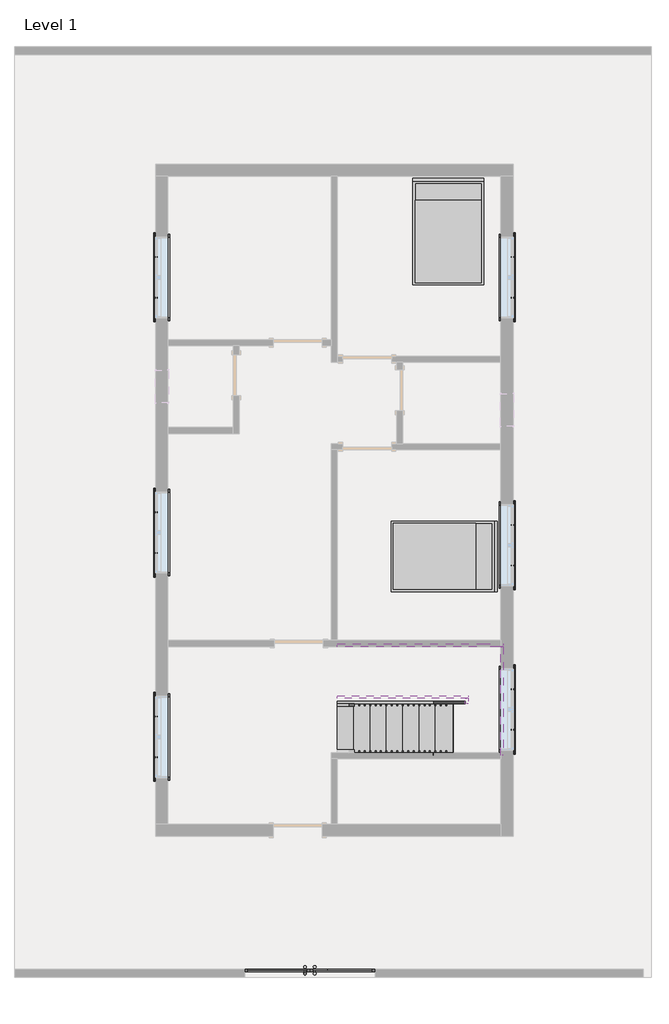
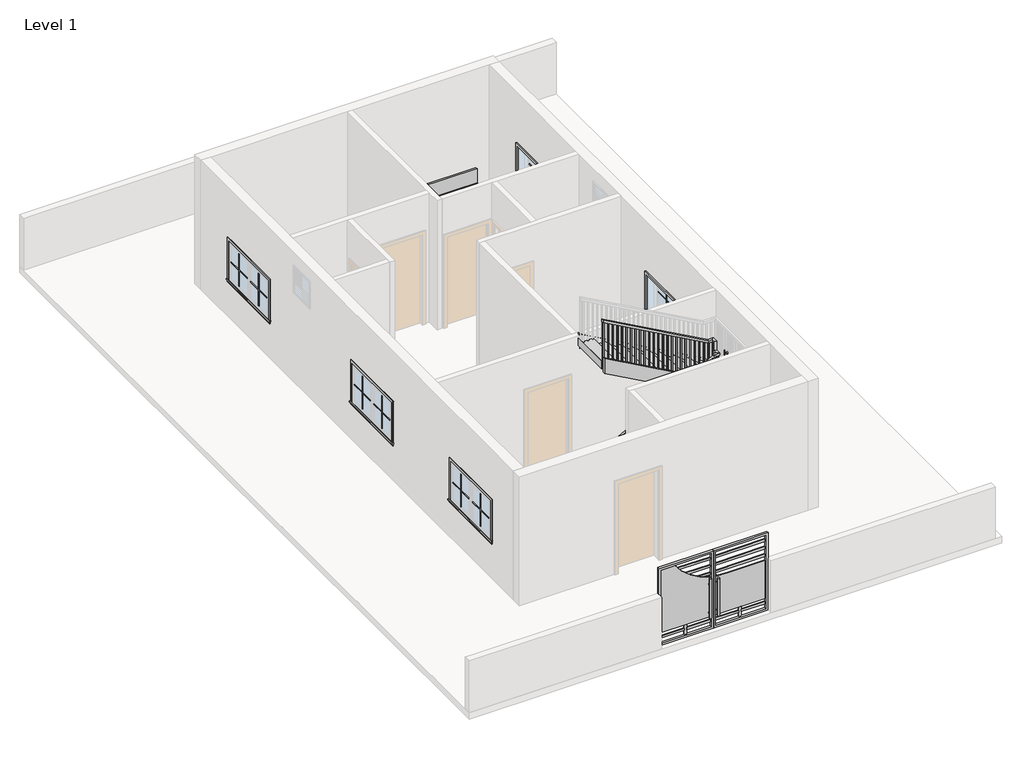
# One storey, part 3 of 3: 25 proxies, 6 members, 2 furniture elements, 1 railing, 1 stair flight.
"""IFC4 building model written with IfcOpenShell, lengths in millimetres."""

from ifc_helpers import new_model, si_unit, frame, origin, place, context, project, spatial, polyline, outline, extrude, faceted_brep, transform, mapped, element, save
from components import generic_models_113f6068, muntin_pattern_2x2_muntin_pattern_2x2_9352d081, muntin_pattern_2x2_muntin_pattern_2x2_5c2cbe28, trim_window_exterior_flat_with_sill_979bde60, trim_window_interior_flat_picture_frame_7883d11b, bed_17739_bed_17739_15c61121, stair_flight_11d7aa5f

model = new_model("IFC4")

# Units and contexts
model_context = context("Model", 3, world=origin())
ifc_project = project(units=[si_unit("LENGTHUNIT", "METRE", prefix="MILLI")], contexts=[model_context])

# Site, building, storey
site = spatial("IfcSite", under=ifc_project)
building = spatial("IfcBuilding", under=site)
storey = spatial("IfcBuildingStorey", under=building, Name="Level 1", Elevation=0.0)

# Proxies
placement = place(None, origin())
generic_models_shape = generic_models_113f6068(model_context)
element("IfcBuildingElementProxy", 1, Name="Generic Models", at=placement, inside=storey, context=model_context, shape_type="MappedRepresentation", body=[
    mapped(generic_models_shape, transform((-1712.32188, -8858.1500287, 0.0), x_axis=(1.0, 0.0, 0.0), y_axis=(0.0, 1.0, 0.0), z_axis=(0.0, 0.0, 1.0))),
])
muntin_pattern_2x2_muntin_pattern_2x2_shape = muntin_pattern_2x2_muntin_pattern_2x2_9352d081(model_context)
element("IfcBuildingElementProxy", 2, Name="Muntin Pattern_2x2 : Muntin Pattern_2x2", ObjectType="Muntin Pattern_2x2 : Muntin Pattern_2x2", at=placement, inside=storey, context=model_context, shape_type="MappedRepresentation", body=[
    mapped(muntin_pattern_2x2_muntin_pattern_2x2_shape, transform((-4579.34688, 3675.02881, 984.25), x_axis=(0.0, 1.0, 0.0), y_axis=(-1.0, 0.0, 0.0), z_axis=(0.0, 0.0, 1.0))),
])
element("IfcBuildingElementProxy", 3, Name="Muntin Pattern_2x2 : Muntin Pattern_2x2", ObjectType="Muntin Pattern_2x2 : Muntin Pattern_2x2", at=placement, inside=storey, context=model_context, shape_type="MappedRepresentation", body=[
    mapped(muntin_pattern_2x2_muntin_pattern_2x2_shape, transform((-4579.34688, -1087.47119, 984.25), x_axis=(0.0, 1.0, 0.0), y_axis=(-1.0, 0.0, 0.0), z_axis=(0.0, 0.0, 1.0))),
])
element("IfcBuildingElementProxy", 4, Name="Muntin Pattern_2x2 : Muntin Pattern_2x2", ObjectType="Muntin Pattern_2x2 : Muntin Pattern_2x2", at=placement, inside=storey, context=model_context, shape_type="MappedRepresentation", body=[
    mapped(muntin_pattern_2x2_muntin_pattern_2x2_shape, transform((-4579.34688, -4900.64619, 984.25), x_axis=(0.0, 1.0, 0.0), y_axis=(-1.0, 0.0, 0.0), z_axis=(0.0, 0.0, 1.0))),
])
element("IfcBuildingElementProxy", 5, Name="Muntin Pattern_2x2 : Muntin Pattern_2x2", ObjectType="Muntin Pattern_2x2 : Muntin Pattern_2x2", at=placement, inside=storey, context=model_context, shape_type="MappedRepresentation", body=[
    mapped(muntin_pattern_2x2_muntin_pattern_2x2_shape, transform((2069.10312, -3630.64619, 984.25), x_axis=(0.0, -1.0, 0.0), y_axis=(1.0, 0.0, 0.0), z_axis=(0.0, 0.0, 1.0))),
])
element("IfcBuildingElementProxy", 6, Name="Muntin Pattern_2x2 : Muntin Pattern_2x2", ObjectType="Muntin Pattern_2x2 : Muntin Pattern_2x2", at=placement, inside=storey, context=model_context, shape_type="MappedRepresentation", body=[
    mapped(muntin_pattern_2x2_muntin_pattern_2x2_shape, transform((2069.10312, 4433.85381, 984.25), x_axis=(0.0, -1.0, 0.0), y_axis=(1.0, 0.0, 0.0), z_axis=(0.0, 0.0, 1.0))),
])
element("IfcBuildingElementProxy", 7, Name="Muntin Pattern_2x2 : Muntin Pattern_2x2", ObjectType="Muntin Pattern_2x2 : Muntin Pattern_2x2", at=placement, inside=storey, context=model_context, shape_type="MappedRepresentation", body=[
    mapped(muntin_pattern_2x2_muntin_pattern_2x2_shape, transform((2069.10312, -563.59619, 984.25), x_axis=(0.0, -1.0, 0.0), y_axis=(1.0, 0.0, 0.0), z_axis=(0.0, 0.0, 1.0))),
])
muntin_pattern_2x2_muntin_pattern_2x2_2_shape = muntin_pattern_2x2_muntin_pattern_2x2_5c2cbe28(model_context)
element("IfcBuildingElementProxy", 8, Name="Muntin Pattern_2x2 : Muntin Pattern_2x2", ObjectType="Muntin Pattern_2x2 : Muntin Pattern_2x2", at=placement, inside=storey, context=model_context, shape_type="MappedRepresentation", body=[
    mapped(muntin_pattern_2x2_muntin_pattern_2x2_2_shape, transform((-4579.34688, 4433.85381, 984.25), x_axis=(0.0, -1.0, 0.0), y_axis=(1.0, 0.0, 0.0), z_axis=(0.0, 0.0, 1.0))),
])
element("IfcBuildingElementProxy", 9, Name="Muntin Pattern_2x2 : Muntin Pattern_2x2", ObjectType="Muntin Pattern_2x2 : Muntin Pattern_2x2", at=placement, inside=storey, context=model_context, shape_type="MappedRepresentation", body=[
    mapped(muntin_pattern_2x2_muntin_pattern_2x2_2_shape, transform((-4579.34688, -328.64619, 984.25), x_axis=(0.0, -1.0, 0.0), y_axis=(1.0, 0.0, 0.0), z_axis=(0.0, 0.0, 1.0))),
])
element("IfcBuildingElementProxy", 10, Name="Muntin Pattern_2x2 : Muntin Pattern_2x2", ObjectType="Muntin Pattern_2x2 : Muntin Pattern_2x2", at=placement, inside=storey, context=model_context, shape_type="MappedRepresentation", body=[
    mapped(muntin_pattern_2x2_muntin_pattern_2x2_2_shape, transform((-4579.34688, -4141.82119, 984.25), x_axis=(0.0, -1.0, 0.0), y_axis=(1.0, 0.0, 0.0), z_axis=(0.0, 0.0, 1.0))),
])
element("IfcBuildingElementProxy", 11, Name="Muntin Pattern_2x2 : Muntin Pattern_2x2", ObjectType="Muntin Pattern_2x2 : Muntin Pattern_2x2", at=placement, inside=storey, context=model_context, shape_type="MappedRepresentation", body=[
    mapped(muntin_pattern_2x2_muntin_pattern_2x2_2_shape, transform((2069.10312, -4389.47119, 984.25), x_axis=(0.0, 1.0, 0.0), y_axis=(-1.0, 0.0, 0.0), z_axis=(0.0, 0.0, 1.0))),
])
element("IfcBuildingElementProxy", 12, Name="Muntin Pattern_2x2 : Muntin Pattern_2x2", ObjectType="Muntin Pattern_2x2 : Muntin Pattern_2x2", at=placement, inside=storey, context=model_context, shape_type="MappedRepresentation", body=[
    mapped(muntin_pattern_2x2_muntin_pattern_2x2_2_shape, transform((2069.10312, 3675.02881, 984.25), x_axis=(0.0, 1.0, 0.0), y_axis=(-1.0, 0.0, 0.0), z_axis=(0.0, 0.0, 1.0))),
])
element("IfcBuildingElementProxy", 13, Name="Muntin Pattern_2x2 : Muntin Pattern_2x2", ObjectType="Muntin Pattern_2x2 : Muntin Pattern_2x2", at=placement, inside=storey, context=model_context, shape_type="MappedRepresentation", body=[
    mapped(muntin_pattern_2x2_muntin_pattern_2x2_2_shape, transform((2069.10312, -1322.42119, 984.25), x_axis=(0.0, 1.0, 0.0), y_axis=(-1.0, 0.0, 0.0), z_axis=(0.0, 0.0, 1.0))),
])
trim_window_exterior_flat_with_sill_shape = trim_window_exterior_flat_with_sill_979bde60(model_context)
element("IfcBuildingElementProxy", 14, Name="Trim-Window-Exterior-Flat : with Sill", ObjectType="Trim-Window-Exterior-Flat : with Sill", at=placement, inside=storey, context=model_context, shape_type="MappedRepresentation", body=[
    mapped(trim_window_exterior_flat_with_sill_shape, transform((-4588.87188, 4054.44131, 1828.8), x_axis=(0.0, -1.0, 0.0), y_axis=(0.0, 0.0, 1.0), z_axis=(-1.0, 0.0, 0.0))),
])
element("IfcBuildingElementProxy", 15, Name="Trim-Window-Exterior-Flat : with Sill", ObjectType="Trim-Window-Exterior-Flat : with Sill", at=placement, inside=storey, context=model_context, shape_type="MappedRepresentation", body=[
    mapped(trim_window_exterior_flat_with_sill_shape, transform((-4588.87188, -708.05869, 1828.8), x_axis=(0.0, -1.0, 0.0), y_axis=(0.0, 0.0, 1.0), z_axis=(-1.0, 0.0, 0.0))),
])
element("IfcBuildingElementProxy", 16, Name="Trim-Window-Exterior-Flat : with Sill", ObjectType="Trim-Window-Exterior-Flat : with Sill", at=placement, inside=storey, context=model_context, shape_type="MappedRepresentation", body=[
    mapped(trim_window_exterior_flat_with_sill_shape, transform((-4588.87188, -4521.23369, 1828.8), x_axis=(0.0, -1.0, 0.0), y_axis=(0.0, 0.0, 1.0), z_axis=(-1.0, 0.0, 0.0))),
])
element("IfcBuildingElementProxy", 17, Name="Trim-Window-Exterior-Flat : with Sill", ObjectType="Trim-Window-Exterior-Flat : with Sill", at=placement, inside=storey, context=model_context, shape_type="MappedRepresentation", body=[
    mapped(trim_window_exterior_flat_with_sill_shape, transform((2078.62812, -4010.05869, 1828.8), x_axis=(0.0, 1.0, 0.0), y_axis=(0.0, 0.0, 1.0), z_axis=(1.0, 0.0, 0.0))),
])
element("IfcBuildingElementProxy", 18, Name="Trim-Window-Exterior-Flat : with Sill", ObjectType="Trim-Window-Exterior-Flat : with Sill", at=placement, inside=storey, context=model_context, shape_type="MappedRepresentation", body=[
    mapped(trim_window_exterior_flat_with_sill_shape, transform((2078.62812, 4054.44131, 1828.8), x_axis=(0.0, 1.0, 0.0), y_axis=(0.0, 0.0, 1.0), z_axis=(1.0, 0.0, 0.0))),
])
element("IfcBuildingElementProxy", 19, Name="Trim-Window-Exterior-Flat : with Sill", ObjectType="Trim-Window-Exterior-Flat : with Sill", at=placement, inside=storey, context=model_context, shape_type="MappedRepresentation", body=[
    mapped(trim_window_exterior_flat_with_sill_shape, transform((2078.62812, -943.00869, 1828.8), x_axis=(0.0, 1.0, 0.0), y_axis=(0.0, 0.0, 1.0), z_axis=(1.0, 0.0, 0.0))),
])
trim_window_interior_flat_picture_frame_shape = trim_window_interior_flat_picture_frame_7883d11b(model_context)
element("IfcBuildingElementProxy", 20, Name="Trim-Window-Interior-Flat : Picture Frame", ObjectType="Trim-Window-Interior-Flat : Picture Frame", at=placement, inside=storey, context=model_context, shape_type="MappedRepresentation", body=[
    mapped(trim_window_interior_flat_picture_frame_shape, transform((-4360.27188, 4054.44131, 1828.8), x_axis=(0.0, 1.0, 0.0), y_axis=(0.0, 0.0, 1.0), z_axis=(1.0, 0.0, 0.0))),
])
element("IfcBuildingElementProxy", 21, Name="Trim-Window-Interior-Flat : Picture Frame", ObjectType="Trim-Window-Interior-Flat : Picture Frame", at=placement, inside=storey, context=model_context, shape_type="MappedRepresentation", body=[
    mapped(trim_window_interior_flat_picture_frame_shape, transform((-4360.27188, -708.05869, 1828.8), x_axis=(0.0, 1.0, 0.0), y_axis=(0.0, 0.0, 1.0), z_axis=(1.0, 0.0, 0.0))),
])
element("IfcBuildingElementProxy", 22, Name="Trim-Window-Interior-Flat : Picture Frame", ObjectType="Trim-Window-Interior-Flat : Picture Frame", at=placement, inside=storey, context=model_context, shape_type="MappedRepresentation", body=[
    mapped(trim_window_interior_flat_picture_frame_shape, transform((-4360.27188, -4521.23369, 1828.8), x_axis=(0.0, 1.0, 0.0), y_axis=(0.0, 0.0, 1.0), z_axis=(1.0, 0.0, 0.0))),
])
element("IfcBuildingElementProxy", 23, Name="Trim-Window-Interior-Flat : Picture Frame", ObjectType="Trim-Window-Interior-Flat : Picture Frame", at=placement, inside=storey, context=model_context, shape_type="MappedRepresentation", body=[
    mapped(trim_window_interior_flat_picture_frame_shape, transform((1850.02812, -4010.05869, 1828.8), x_axis=(0.0, -1.0, 0.0), y_axis=(0.0, 0.0, 1.0), z_axis=(-1.0, 0.0, 0.0))),
])
element("IfcBuildingElementProxy", 24, Name="Trim-Window-Interior-Flat : Picture Frame", ObjectType="Trim-Window-Interior-Flat : Picture Frame", at=placement, inside=storey, context=model_context, shape_type="MappedRepresentation", body=[
    mapped(trim_window_interior_flat_picture_frame_shape, transform((1850.02812, 4054.44131, 1828.8), x_axis=(0.0, -1.0, 0.0), y_axis=(0.0, 0.0, 1.0), z_axis=(-1.0, 0.0, 0.0))),
])
element("IfcBuildingElementProxy", 25, Name="Trim-Window-Interior-Flat : Picture Frame", ObjectType="Trim-Window-Interior-Flat : Picture Frame", at=placement, inside=storey, context=model_context, shape_type="MappedRepresentation", body=[
    mapped(trim_window_interior_flat_picture_frame_shape, transform((1850.02812, -943.00869, 1828.8), x_axis=(0.0, -1.0, 0.0), y_axis=(0.0, 0.0, 1.0), z_axis=(-1.0, 0.0, 0.0))),
])

# Furniture
bed_17739_bed_17739_shape = bed_17739_bed_17739_15c61121(model_context)
element("IfcFurniture", 26, ObjectType="Bed_17739 : Bed_17739", at=placement, inside=storey, context=model_context, shape_type="MappedRepresentation", body=[
    mapped(bed_17739_bed_17739_shape, transform((872.12812, 4886.29131, 0.0), x_axis=(1.0, 0.0, 0.0), y_axis=(0.0, 1.0, 0.0), z_axis=(0.0, 0.0, 1.0))),
])
element("IfcFurniture", 27, ObjectType="Bed_17739 : Bed_17739", at=placement, inside=storey, context=model_context, shape_type="MappedRepresentation", body=[
    mapped(bed_17739_bed_17739_shape, transform((770.52812, -1152.55869, 0.0), x_axis=(0.0, -1.0, 0.0), y_axis=(1.0, 0.0, 0.0), z_axis=(0.0, 0.0, 1.0))),
])

# Members
element("IfcMember", 28, ObjectType="Stringer - 2\" Width", at=placement, inside=storey, context=model_context, shape_type="SweptSolid", body=[
    extrude(outline(polyline([(207.5983948, -1197.97188), (0.0, -1197.97188), (0.0, -944.0273772), (1185.3641651, 1189.62812), (1534.0428392, 1189.62812), (207.5983948, -1197.97188)])), frame((0.0, -3902.10869, 0.0), z_axis=(0.0, 1.0, 0.0), x_axis=(0.0, 0.0, 1.0)), (0.0, 0.0, 1.0), 50.8),
])
element("IfcMember", 29, ObjectType="Stringer - 2\" Width", at=placement, inside=storey, context=model_context, shape_type="SweptSolid", body=[
    extrude(outline(polyline([(1240.42812, -3902.10869), (1189.62812, -3902.10869), (1189.62812, -3800.50869), (1240.42812, -3800.50869), (1240.42812, -3902.10869)])), frame((0.0, 0.0, 1295.4), z_axis=(0.0, 0.0, 1.0), x_axis=(1.0, 0.0, 0.0)), (0.0, 0.0, 1.0), 304.8),
])
element("IfcMember", 30, ObjectType="Stringer - 2\" Width", at=placement, inside=storey, context=model_context, shape_type="SweptSolid", body=[
    extrude(outline(polyline([(1382.9197207, 1240.42812), (1731.5983948, 1240.42812), (3086.2650614, -1197.97188), (2737.5863873, -1197.97188), (1382.9197207, 1240.42812)])), frame((0.0, -3800.50869, 0.0), z_axis=(0.0, 1.0, 0.0), x_axis=(0.0, 0.0, 1.0)), (0.0, 0.0, 1.0), 50.8),
])
element("IfcMember", 31, ObjectType="Stringer - 2\" Width", at=placement, inside=storey, context=model_context, shape_type="SweptSolid", body=[
    extrude(outline(polyline([(207.5983948, -1197.97188), (0.0, -1197.97188), (0.0, -944.0273772), (1552.253054, 1850.02812), (1600.2, 1850.02812), (1600.2, 1308.7110094), (207.5983948, -1197.97188)])), frame((0.0, -4867.30869, 0.0), z_axis=(0.0, 1.0, 0.0), x_axis=(0.0, 0.0, 1.0)), (0.0, 0.0, 1.0), 50.8),
])
element("IfcMember", 32, ObjectType="Stringer - 2\" Width", at=placement, inside=storey, context=model_context, shape_type="SweptSolid", body=[
    extrude(outline(polyline([(1900.82812, -4867.30869), (1850.02812, -4867.30869), (1850.02812, -2835.30869), (1900.82812, -2835.30869), (1900.82812, -4867.30869)])), frame((0.0, 0.0, 1295.4), z_axis=(0.0, 0.0, 1.0), x_axis=(1.0, 0.0, 0.0)), (0.0, 0.0, 1.0), 304.8),
])
element("IfcMember", 33, ObjectType="Stringer - 2\" Width", at=placement, inside=storey, context=model_context, shape_type="SweptSolid", body=[
    extrude(outline(polyline([(1295.4, 1900.82812), (1364.7095059, 1900.82812), (3086.2650614, -1197.97188), (2737.5863873, -1197.97188), (1295.4, 1397.9636172), (1295.4, 1900.82812)])), frame((0.0, -2835.30869, 0.0), z_axis=(0.0, 1.0, 0.0), x_axis=(0.0, 0.0, 1.0)), (0.0, 0.0, 1.0), 50.8),
])

# Railing
element("IfcRailing", 34, ObjectType="Handrail - Rectangular", at=placement, inside=storey, context=model_context, shape_type="SolidModel", body=[
    faceted_brep([(-1197.97188, -3902.10869, 1083.7333333), (-1197.97188, -3902.10869, 1025.620221), (-1197.97188, -3952.90869, 1025.620221), (-1197.97188, -3952.90869, 1083.7333333), (1164.22812, -3902.10869, 2396.0666667), (1215.02812, -3902.10869, 2366.1757765), (1215.02812, -3952.90869, 2366.1757765), (1164.22812, -3952.90869, 2396.0666667), (1164.22812, -3902.10869, 2438.4), (1215.02812, -3902.10869, 2387.6), (1215.02812, -3952.90869, 2387.6), (1164.22812, -3952.90869, 2438.4), (1240.42812, -3902.10869, 2438.4), (1240.42812, -3902.10869, 2387.6), (1291.22812, -3952.90869, 2387.6), (1291.22812, -3952.90869, 2438.4), (1240.42812, -3825.90869, 2438.4), (1240.42812, -3775.10869, 2387.6), (1291.22812, -3775.10869, 2387.6), (1291.22812, -3825.90869, 2438.4), (1240.42812, -3825.90869, 2650.0666667), (1240.42812, -3775.10869, 2599.2666667), (1291.22812, -3775.10869, 2599.2666667), (1291.22812, -3825.90869, 2650.0666667), (1240.42812, -3749.70869, 2650.0666667), (1240.42812, -3749.70869, 2599.2666667), (1291.22812, -3698.90869, 2599.2666667), (1291.22812, -3698.90869, 2650.0666667), (1164.22812, -3749.70869, 2650.0666667), (1151.0645177, -3749.70869, 2599.2666667), (1151.0645177, -3698.90869, 2599.2666667), (1164.22812, -3698.90869, 2650.0666667), (-1197.97188, -3749.70869, 3962.4), (-1197.97188, -3698.90869, 3962.4), (-1197.97188, -3698.90869, 3904.2868876), (-1197.97188, -3749.70869, 3904.2868876)], [[[0, 1, 2, 3]], [[1, 0, 4, 5]], [[2, 1, 5, 6]], [[3, 2, 6, 7]], [[0, 3, 7, 4]], [[5, 4, 8, 9]], [[6, 5, 9, 10]], [[7, 6, 10, 11]], [[4, 7, 11, 8]], [[9, 8, 12, 13]], [[10, 9, 13, 14]], [[11, 10, 14, 15]], [[8, 11, 15, 12]], [[13, 12, 16, 17]], [[14, 13, 17, 18]], [[15, 14, 18, 19]], [[12, 15, 19, 16]], [[17, 16, 20, 21]], [[18, 17, 21, 22]], [[19, 18, 22, 23]], [[16, 19, 23, 20]], [[21, 20, 24, 25]], [[22, 21, 25, 26]], [[23, 22, 26, 27]], [[20, 23, 27, 24]], [[25, 24, 28, 29]], [[26, 25, 29, 30]], [[27, 26, 30, 31]], [[24, 27, 31, 28]], [[32, 33, 34, 35]], [[29, 28, 32, 35]], [[30, 29, 35, 34]], [[31, 30, 34, 33]], [[28, 31, 33, 32]]]),
    extrude(outline(polyline([(3895.4674432, -1182.09688), (2878.6666667, -1182.09688), (2878.6666667, -1163.04688), (3884.8841099, -1163.04688), (3895.4674432, -1182.09688)])), frame((0.0, -3733.83369, 0.0), z_axis=(0.0, 1.0, 0.0), x_axis=(0.0, 0.0, 1.0)), (0.0, 0.0, 1.0), 19.05),
    extrude(outline(polyline([(3839.0229988, -1080.49688), (2878.6666667, -1080.49688), (2878.6666667, -1061.44688), (3828.4396654, -1061.44688), (3839.0229988, -1080.49688)])), frame((0.0, -3733.83369, 0.0), z_axis=(0.0, 1.0, 0.0), x_axis=(0.0, 0.0, 1.0)), (0.0, 0.0, 1.0), 19.05),
    extrude(outline(polyline([(3782.5785543, -978.89688), (2878.6666667, -978.89688), (2878.6666667, -959.84688), (3771.995221, -959.84688), (3782.5785543, -978.89688)])), frame((0.0, -3733.83369, 0.0), z_axis=(0.0, 1.0, 0.0), x_axis=(0.0, 0.0, 1.0)), (0.0, 0.0, 1.0), 19.05),
    extrude(outline(polyline([(3726.1341099, -877.29688), (2709.3333333, -877.29688), (2709.3333333, -858.24688), (3715.5507765, -858.24688), (3726.1341099, -877.29688)])), frame((0.0, -3733.83369, 0.0), z_axis=(0.0, 1.0, 0.0), x_axis=(0.0, 0.0, 1.0)), (0.0, 0.0, 1.0), 19.05),
    extrude(outline(polyline([(3669.6896654, -775.69688), (2709.3333333, -775.69688), (2709.3333333, -756.64688), (3659.1063321, -756.64688), (3669.6896654, -775.69688)])), frame((0.0, -3733.83369, 0.0), z_axis=(0.0, 1.0, 0.0), x_axis=(0.0, 0.0, 1.0)), (0.0, 0.0, 1.0), 19.05),
    extrude(outline(polyline([(3613.245221, -674.09688), (2709.3333333, -674.09688), (2709.3333333, -655.04688), (3602.6618876, -655.04688), (3613.245221, -674.09688)])), frame((0.0, -3733.83369, 0.0), z_axis=(0.0, 1.0, 0.0), x_axis=(0.0, 0.0, 1.0)), (0.0, 0.0, 1.0), 19.05),
    extrude(outline(polyline([(3556.8007765, -572.49688), (2540.0, -572.49688), (2540.0, -553.44688), (3546.2174432, -553.44688), (3556.8007765, -572.49688)])), frame((0.0, -3733.83369, 0.0), z_axis=(0.0, 1.0, 0.0), x_axis=(0.0, 0.0, 1.0)), (0.0, 0.0, 1.0), 19.05),
    extrude(outline(polyline([(3500.3563321, -470.89688), (2540.0, -470.89688), (2540.0, -451.84688), (3489.7729988, -451.84688), (3500.3563321, -470.89688)])), frame((0.0, -3733.83369, 0.0), z_axis=(0.0, 1.0, 0.0), x_axis=(0.0, 0.0, 1.0)), (0.0, 0.0, 1.0), 19.05),
    extrude(outline(polyline([(3443.9118876, -369.29688), (2540.0, -369.29688), (2540.0, -350.24688), (3433.3285543, -350.24688), (3443.9118876, -369.29688)])), frame((0.0, -3733.83369, 0.0), z_axis=(0.0, 1.0, 0.0), x_axis=(0.0, 0.0, 1.0)), (0.0, 0.0, 1.0), 19.05),
    extrude(outline(polyline([(3387.4674432, -267.69688), (2370.6666667, -267.69688), (2370.6666667, -248.64688), (3376.8841099, -248.64688), (3387.4674432, -267.69688)])), frame((0.0, -3733.83369, 0.0), z_axis=(0.0, 1.0, 0.0), x_axis=(0.0, 0.0, 1.0)), (0.0, 0.0, 1.0), 19.05),
    extrude(outline(polyline([(3331.0229988, -166.09688), (2370.6666667, -166.09688), (2370.6666667, -147.04688), (3320.4396654, -147.04688), (3331.0229988, -166.09688)])), frame((0.0, -3733.83369, 0.0), z_axis=(0.0, 1.0, 0.0), x_axis=(0.0, 0.0, 1.0)), (0.0, 0.0, 1.0), 19.05),
    extrude(outline(polyline([(3274.5785543, -64.49688), (2370.6666667, -64.49688), (2370.6666667, -45.44688), (3263.995221, -45.44688), (3274.5785543, -64.49688)])), frame((0.0, -3733.83369, 0.0), z_axis=(0.0, 1.0, 0.0), x_axis=(0.0, 0.0, 1.0)), (0.0, 0.0, 1.0), 19.05),
    extrude(outline(polyline([(3218.1341099, 37.10312), (2201.3333333, 37.10312), (2201.3333333, 56.15312), (3207.5507765, 56.15312), (3218.1341099, 37.10312)])), frame((0.0, -3733.83369, 0.0), z_axis=(0.0, 1.0, 0.0), x_axis=(0.0, 0.0, 1.0)), (0.0, 0.0, 1.0), 19.05),
    extrude(outline(polyline([(3161.6896654, 138.70312), (2201.3333333, 138.70312), (2201.3333333, 157.75312), (3151.1063321, 157.75312), (3161.6896654, 138.70312)])), frame((0.0, -3733.83369, 0.0), z_axis=(0.0, 1.0, 0.0), x_axis=(0.0, 0.0, 1.0)), (0.0, 0.0, 1.0), 19.05),
    extrude(outline(polyline([(3105.245221, 240.30312), (2201.3333333, 240.30312), (2201.3333333, 259.35312), (3094.6618876, 259.35312), (3105.245221, 240.30312)])), frame((0.0, -3733.83369, 0.0), z_axis=(0.0, 1.0, 0.0), x_axis=(0.0, 0.0, 1.0)), (0.0, 0.0, 1.0), 19.05),
    extrude(outline(polyline([(3048.8007765, 341.90312), (2032.0, 341.90312), (2032.0, 360.95312), (3038.2174432, 360.95312), (3048.8007765, 341.90312)])), frame((0.0, -3733.83369, 0.0), z_axis=(0.0, 1.0, 0.0), x_axis=(0.0, 0.0, 1.0)), (0.0, 0.0, 1.0), 19.05),
    extrude(outline(polyline([(2992.3563321, 443.50312), (2032.0, 443.50312), (2032.0, 462.55312), (2981.7729988, 462.55312), (2992.3563321, 443.50312)])), frame((0.0, -3733.83369, 0.0), z_axis=(0.0, 1.0, 0.0), x_axis=(0.0, 0.0, 1.0)), (0.0, 0.0, 1.0), 19.05),
    extrude(outline(polyline([(2935.9118876, 545.10312), (2032.0, 545.10312), (2032.0, 564.15312), (2925.3285543, 564.15312), (2935.9118876, 545.10312)])), frame((0.0, -3733.83369, 0.0), z_axis=(0.0, 1.0, 0.0), x_axis=(0.0, 0.0, 1.0)), (0.0, 0.0, 1.0), 19.05),
    extrude(outline(polyline([(2879.4674432, 646.70312), (1862.6666667, 646.70312), (1862.6666667, 665.75312), (2868.8841099, 665.75312), (2879.4674432, 646.70312)])), frame((0.0, -3733.83369, 0.0), z_axis=(0.0, 1.0, 0.0), x_axis=(0.0, 0.0, 1.0)), (0.0, 0.0, 1.0), 19.05),
    extrude(outline(polyline([(2823.0229988, 748.30312), (1862.6666667, 748.30312), (1862.6666667, 767.35312), (2812.4396654, 767.35312), (2823.0229988, 748.30312)])), frame((0.0, -3733.83369, 0.0), z_axis=(0.0, 1.0, 0.0), x_axis=(0.0, 0.0, 1.0)), (0.0, 0.0, 1.0), 19.05),
    extrude(outline(polyline([(2766.5785543, 849.90312), (1862.6666667, 849.90312), (1862.6666667, 868.95312), (2755.995221, 868.95312), (2766.5785543, 849.90312)])), frame((0.0, -3733.83369, 0.0), z_axis=(0.0, 1.0, 0.0), x_axis=(0.0, 0.0, 1.0)), (0.0, 0.0, 1.0), 19.05),
    extrude(outline(polyline([(2710.1341099, 951.50312), (1693.3333333, 951.50312), (1693.3333333, 970.55312), (2699.5507765, 970.55312), (2710.1341099, 951.50312)])), frame((0.0, -3733.83369, 0.0), z_axis=(0.0, 1.0, 0.0), x_axis=(0.0, 0.0, 1.0)), (0.0, 0.0, 1.0), 19.05),
    extrude(outline(polyline([(2653.6896654, 1053.10312), (1693.3333333, 1053.10312), (1693.3333333, 1072.15312), (2643.1063321, 1072.15312), (2653.6896654, 1053.10312)])), frame((0.0, -3733.83369, 0.0), z_axis=(0.0, 1.0, 0.0), x_axis=(0.0, 0.0, 1.0)), (0.0, 0.0, 1.0), 19.05),
    extrude(outline(polyline([(2597.245221, 1154.70312), (1693.3333333, 1154.70312), (1693.3333333, 1173.75312), (2586.6618876, 1173.75312), (2597.245221, 1154.70312)])), frame((0.0, -3733.83369, 0.0), z_axis=(0.0, 1.0, 0.0), x_axis=(0.0, 0.0, 1.0)), (0.0, 0.0, 1.0), 19.05),
    extrude(outline(polyline([(1256.30312, -3835.43369), (1256.30312, -3816.38369), (1275.35312, -3816.38369), (1275.35312, -3835.43369), (1256.30312, -3835.43369)])), frame((0.0, 0.0, 1524.0), z_axis=(0.0, 0.0, 1.0), x_axis=(1.0, 0.0, 0.0)), (0.0, 0.0, 1.0), 863.6),
    extrude(outline(polyline([(1230.90312, -3917.98369), (1249.95312, -3917.98369), (1249.95312, -3937.03369), (1230.90312, -3937.03369), (1230.90312, -3917.98369)])), frame((0.0, 0.0, 1524.0), z_axis=(0.0, 0.0, 1.0), x_axis=(1.0, 0.0, 0.0)), (0.0, 0.0, 1.0), 863.6),
    extrude(outline(polyline([(2318.5507765, 1129.30312), (1354.6666667, 1129.30312), (1354.6666667, 1148.35312), (2329.1341099, 1148.35312), (2318.5507765, 1129.30312)])), frame((0.0, -3937.03369, 0.0), z_axis=(0.0, 1.0, 0.0), x_axis=(0.0, 0.0, 1.0)), (0.0, 0.0, 1.0), 19.05),
    extrude(outline(polyline([(2262.1063321, 1027.70312), (1354.6666667, 1027.70312), (1354.6666667, 1046.75312), (2272.6896654, 1046.75312), (2262.1063321, 1027.70312)])), frame((0.0, -3937.03369, 0.0), z_axis=(0.0, 1.0, 0.0), x_axis=(0.0, 0.0, 1.0)), (0.0, 0.0, 1.0), 19.05),
    extrude(outline(polyline([(2205.6618876, 926.10312), (1354.6666667, 926.10312), (1354.6666667, 945.15312), (2216.245221, 945.15312), (2205.6618876, 926.10312)])), frame((0.0, -3937.03369, 0.0), z_axis=(0.0, 1.0, 0.0), x_axis=(0.0, 0.0, 1.0)), (0.0, 0.0, 1.0), 19.05),
    extrude(outline(polyline([(2149.2174432, 824.50312), (1185.3333333, 824.50312), (1185.3333333, 843.55312), (2159.8007765, 843.55312), (2149.2174432, 824.50312)])), frame((0.0, -3937.03369, 0.0), z_axis=(0.0, 1.0, 0.0), x_axis=(0.0, 0.0, 1.0)), (0.0, 0.0, 1.0), 19.05),
    extrude(outline(polyline([(2092.7729988, 722.90312), (1185.3333333, 722.90312), (1185.3333333, 741.95312), (2103.3563321, 741.95312), (2092.7729988, 722.90312)])), frame((0.0, -3937.03369, 0.0), z_axis=(0.0, 1.0, 0.0), x_axis=(0.0, 0.0, 1.0)), (0.0, 0.0, 1.0), 19.05),
    extrude(outline(polyline([(2036.3285543, 621.30312), (1185.3333333, 621.30312), (1185.3333333, 640.35312), (2046.9118876, 640.35312), (2036.3285543, 621.30312)])), frame((0.0, -3937.03369, 0.0), z_axis=(0.0, 1.0, 0.0), x_axis=(0.0, 0.0, 1.0)), (0.0, 0.0, 1.0), 19.05),
    extrude(outline(polyline([(1979.8841099, 519.70312), (1016.0, 519.70312), (1016.0, 538.75312), (1990.4674432, 538.75312), (1979.8841099, 519.70312)])), frame((0.0, -3937.03369, 0.0), z_axis=(0.0, 1.0, 0.0), x_axis=(0.0, 0.0, 1.0)), (0.0, 0.0, 1.0), 19.05),
    extrude(outline(polyline([(1923.4396654, 418.10312), (1016.0, 418.10312), (1016.0, 437.15312), (1934.0229988, 437.15312), (1923.4396654, 418.10312)])), frame((0.0, -3937.03369, 0.0), z_axis=(0.0, 1.0, 0.0), x_axis=(0.0, 0.0, 1.0)), (0.0, 0.0, 1.0), 19.05),
    extrude(outline(polyline([(1866.995221, 316.50312), (1016.0, 316.50312), (1016.0, 335.55312), (1877.5785543, 335.55312), (1866.995221, 316.50312)])), frame((0.0, -3937.03369, 0.0), z_axis=(0.0, 1.0, 0.0), x_axis=(0.0, 0.0, 1.0)), (0.0, 0.0, 1.0), 19.05),
    extrude(outline(polyline([(1810.5507765, 214.90312), (846.6666667, 214.90312), (846.6666667, 233.95312), (1821.1341099, 233.95312), (1810.5507765, 214.90312)])), frame((0.0, -3937.03369, 0.0), z_axis=(0.0, 1.0, 0.0), x_axis=(0.0, 0.0, 1.0)), (0.0, 0.0, 1.0), 19.05),
    extrude(outline(polyline([(1754.1063321, 113.30312), (846.6666667, 113.30312), (846.6666667, 132.35312), (1764.6896654, 132.35312), (1754.1063321, 113.30312)])), frame((0.0, -3937.03369, 0.0), z_axis=(0.0, 1.0, 0.0), x_axis=(0.0, 0.0, 1.0)), (0.0, 0.0, 1.0), 19.05),
    extrude(outline(polyline([(1697.6618876, 11.70312), (846.6666667, 11.70312), (846.6666667, 30.75312), (1708.245221, 30.75312), (1697.6618876, 11.70312)])), frame((0.0, -3937.03369, 0.0), z_axis=(0.0, 1.0, 0.0), x_axis=(0.0, 0.0, 1.0)), (0.0, 0.0, 1.0), 19.05),
    extrude(outline(polyline([(1641.2174432, -89.89688), (677.3333333, -89.89688), (677.3333333, -70.84688), (1651.8007765, -70.84688), (1641.2174432, -89.89688)])), frame((0.0, -3937.03369, 0.0), z_axis=(0.0, 1.0, 0.0), x_axis=(0.0, 0.0, 1.0)), (0.0, 0.0, 1.0), 19.05),
    extrude(outline(polyline([(1584.7729988, -191.49688), (677.3333333, -191.49688), (677.3333333, -172.44688), (1595.3563321, -172.44688), (1584.7729988, -191.49688)])), frame((0.0, -3937.03369, 0.0), z_axis=(0.0, 1.0, 0.0), x_axis=(0.0, 0.0, 1.0)), (0.0, 0.0, 1.0), 19.05),
    extrude(outline(polyline([(1528.3285543, -293.09688), (677.3333333, -293.09688), (677.3333333, -274.04688), (1538.9118876, -274.04688), (1528.3285543, -293.09688)])), frame((0.0, -3937.03369, 0.0), z_axis=(0.0, 1.0, 0.0), x_axis=(0.0, 0.0, 1.0)), (0.0, 0.0, 1.0), 19.05),
    extrude(outline(polyline([(1471.8841099, -394.69688), (508.0, -394.69688), (508.0, -375.64688), (1482.4674432, -375.64688), (1471.8841099, -394.69688)])), frame((0.0, -3937.03369, 0.0), z_axis=(0.0, 1.0, 0.0), x_axis=(0.0, 0.0, 1.0)), (0.0, 0.0, 1.0), 19.05),
    extrude(outline(polyline([(1415.4396654, -496.29688), (508.0, -496.29688), (508.0, -477.24688), (1426.0229988, -477.24688), (1415.4396654, -496.29688)])), frame((0.0, -3937.03369, 0.0), z_axis=(0.0, 1.0, 0.0), x_axis=(0.0, 0.0, 1.0)), (0.0, 0.0, 1.0), 19.05),
    extrude(outline(polyline([(1358.995221, -597.89688), (508.0, -597.89688), (508.0, -578.84688), (1369.5785543, -578.84688), (1358.995221, -597.89688)])), frame((0.0, -3937.03369, 0.0), z_axis=(0.0, 1.0, 0.0), x_axis=(0.0, 0.0, 1.0)), (0.0, 0.0, 1.0), 19.05),
    extrude(outline(polyline([(1302.5507765, -699.49688), (338.6666667, -699.49688), (338.6666667, -680.44688), (1313.1341099, -680.44688), (1302.5507765, -699.49688)])), frame((0.0, -3937.03369, 0.0), z_axis=(0.0, 1.0, 0.0), x_axis=(0.0, 0.0, 1.0)), (0.0, 0.0, 1.0), 19.05),
    extrude(outline(polyline([(1246.1063321, -801.09688), (338.6666667, -801.09688), (338.6666667, -782.04688), (1256.6896654, -782.04688), (1246.1063321, -801.09688)])), frame((0.0, -3937.03369, 0.0), z_axis=(0.0, 1.0, 0.0), x_axis=(0.0, 0.0, 1.0)), (0.0, 0.0, 1.0), 19.05),
    extrude(outline(polyline([(1189.6618876, -902.69688), (338.6666667, -902.69688), (338.6666667, -883.64688), (1200.245221, -883.64688), (1189.6618876, -902.69688)])), frame((0.0, -3937.03369, 0.0), z_axis=(0.0, 1.0, 0.0), x_axis=(0.0, 0.0, 1.0)), (0.0, 0.0, 1.0), 19.05),
    extrude(outline(polyline([(1133.2174432, -1004.29688), (169.3333333, -1004.29688), (169.3333333, -985.24688), (1143.8007765, -985.24688), (1133.2174432, -1004.29688)])), frame((0.0, -3937.03369, 0.0), z_axis=(0.0, 1.0, 0.0), x_axis=(0.0, 0.0, 1.0)), (0.0, 0.0, 1.0), 19.05),
    extrude(outline(polyline([(1076.7729988, -1105.89688), (169.3333333, -1105.89688), (169.3333333, -1086.84688), (1087.3563321, -1086.84688), (1076.7729988, -1105.89688)])), frame((0.0, -3937.03369, 0.0), z_axis=(0.0, 1.0, 0.0), x_axis=(0.0, 0.0, 1.0)), (0.0, 0.0, 1.0), 19.05),
    extrude(outline(polyline([(1256.30312, -3733.83369), (1256.30312, -3714.78369), (1275.35312, -3714.78369), (1275.35312, -3733.83369), (1256.30312, -3733.83369)])), frame((0.0, 0.0, 1524.0), z_axis=(0.0, 0.0, 1.0), x_axis=(1.0, 0.0, 0.0)), (0.0, 0.0, 1.0), 1075.2666667),
    extrude(outline(polyline([(1256.30312, -3917.98369), (1275.35312, -3917.98369), (1275.35312, -3937.03369), (1256.30312, -3937.03369), (1256.30312, -3917.98369)])), frame((0.0, 0.0, 1524.0), z_axis=(0.0, 0.0, 1.0), x_axis=(1.0, 0.0, 0.0)), (0.0, 0.0, 1.0), 863.6),
    extrude(outline(polyline([(3904.2868876, -1197.97188), (2878.6666667, -1197.97188), (2878.6666667, -1178.92188), (3893.7035543, -1178.92188), (3904.2868876, -1197.97188)])), frame((0.0, -3733.83369, 0.0), z_axis=(0.0, 1.0, 0.0), x_axis=(0.0, 0.0, 1.0)), (0.0, 0.0, 1.0), 19.05),
    extrude(outline(polyline([(1025.620221, -1197.97188), (169.3333333, -1197.97188), (169.3333333, -1178.92188), (1036.2035543, -1178.92188), (1025.620221, -1197.97188)])), frame((0.0, -3937.03369, 0.0), z_axis=(0.0, 1.0, 0.0), x_axis=(0.0, 0.0, 1.0)), (0.0, 0.0, 1.0), 19.05),
])

# Stair flight
stair_flight_shape = stair_flight_11d7aa5f(model_context)
element("IfcStairFlight", 35, ObjectType="2\" Tread 1\" Nosing 1/4\" Riser", at=placement, inside=storey, context=model_context, shape_type="MappedRepresentation", body=[
    mapped(stair_flight_shape, transform((0.0, 0.0, 0.0), x_axis=(1.0, 0.0, 0.0), y_axis=(0.0, 1.0, 0.0), z_axis=(0.0, 0.0, 1.0))),
])

save(model, "model.ifc")

# Revit data of these elements
# Type
#   sheet = none
#   pipe = none
#   handal = none
#   faram = none
#   Default Elevation = 0
# Type "Muntin Pattern_2x2 : Muntin Pattern_2x2"
#   Width [instance default] = 4' - 0"
#   Thickness = 0' - 0 1/2"
#   Height [instance default] = 4' - 0"
#   Distance = 0' - 0 3/4"
#   Interior Material [instance default] = none
#   Exterior Material [instance default] = none
#   Default Elevation = 0
# Type "Trim-Window-Exterior-Flat : with Sill"
#   Trim Width = 0' - 2 1/4"
#   Trim Thickness_Picture Frame = 0' - 1 1/4"
#   Trim Thickness_with Sill = 0' - 0 3/4"
#   Sill Thickness = 0' - 1 1/4"
#   Opening Width [instance default] = 2' - 0"
#   Opening Height [instance default] = 3' - 0"
#   Default Elevation = 4' - 0"
#   Sill = yes
#   Picture Frame = no
#   Trim Material [instance default] = none
# Type "Trim-Window-Interior-Flat : Picture Frame"
#   Trim Thickness_Picture Frame = 0' - 1 1/4"
#   Trim Width = 0' - 2 1/4"
#   Trim Thickness_with Sill = 0' - 0 3/4"
#   Sill Thickness = 0' - 1 1/4"
#   Opening Width [instance default] = 2' - 0"
#   Opening Height [instance default] = 3' - 0"
#   Default Elevation = 4' - 0"
#   Sill = no
#   Picture Frame = yes
#   Trim Material [instance default] = none
# Type "Bed_17739 : Bed_17739"
#   Default Elevation = 0
# Type "Handrail - Rectangular"
#   Assembly Code = "C2010400"
#   built-in parameter 1008612 = 0.0416667 (stored number, unit not read)
#   built-in parameter 1008611 = 0.0416667 (stored number, unit not read)
#   built-in parameter 1008609 = 0.333333 (stored number, unit not read)
#   built-in parameter 1008604 = 0.166667 (stored number, unit not read)
#   built-in parameter 1008603 = 0.166667 (stored number, unit not read)
#   Railing Height = 3' - 0"
#   built-in parameter 1008630 = 2
#   built-in parameter 1008610 = 2
#   built-in parameter 1008618 = Baluster - Square : 3/4"
# Element 1 (IfcBuildingElementProxy)
#   Phase Created = New Construction
# Elements 2, 3, 4, 5, 6, 7, 8, 9, 10, 11, 12, 13 (IfcBuildingElementProxy, "Muntin Pattern_2x2 : Muntin Pattern_2x2")
#   Width = 2' - 0 5/8"
#   Height = 2' - 6 1/2"
#   Interior Material = Wood - Stained
#   Exterior Material = Clad - White
#   Phase Created = New Construction
#   Materials on its faces: "Clad - White", "Wood - Stained"
# Elements 14, 15, 16, 17, 18, 19 (IfcBuildingElementProxy, "Trim-Window-Exterior-Flat : with Sill")
#   Opening Width = 5' - 0"
#   Opening Height = 3' - 0"
#   Trim Material = Clad - White
#   Phase Created = New Construction
#   Materials on its faces: "Clad - White"
# Elements 20, 21, 22, 23, 24, 25 (IfcBuildingElementProxy, "Trim-Window-Interior-Flat : Picture Frame")
#   Opening Width = 5' - 0"
#   Opening Height = 3' - 0"
#   Trim Material = Wood - Stained
#   Phase Created = New Construction
#   Materials on its faces: "Wood - Stained"
# Elements 26, 27 (IfcFurniture, "Bed_17739 : Bed_17739")
#   Phase Created = New Construction
#   Materials on its faces: "legs", "sheets", "bed frame", "Blanket"
# Elements 28, 29, 30, 31, 32, 33 (IfcMember, "Stringer - 2\" Width")
#   Phase Created = New Construction
# Element 34 (IfcRailing, "Handrail - Rectangular")
#   Phase Created = New Construction
# Element 35 (IfcStairFlight, "2\" Tread 1\" Nosing 1/4\" Riser")
#   Phase Created = New Construction
# Materials
#   "Clad - White": class "Wood", colour RGB 242 242 238, transparency 0, Cost = 0
#   "Wood - Stained": class "Wood", colour RGB 224 178 126, transparency 0, Cost = 0
#   "legs": colour RGB 90 73 37, transparency 0, Cost = 0
#   "sheets": colour RGB 200 195 176, transparency 0, Cost = 0
#   "bed frame": colour RGB 90 73 37, transparency 0, Cost = 0
#   "Blanket": class "System", colour RGB 59 0 1, transparency 0, Cost = 0
